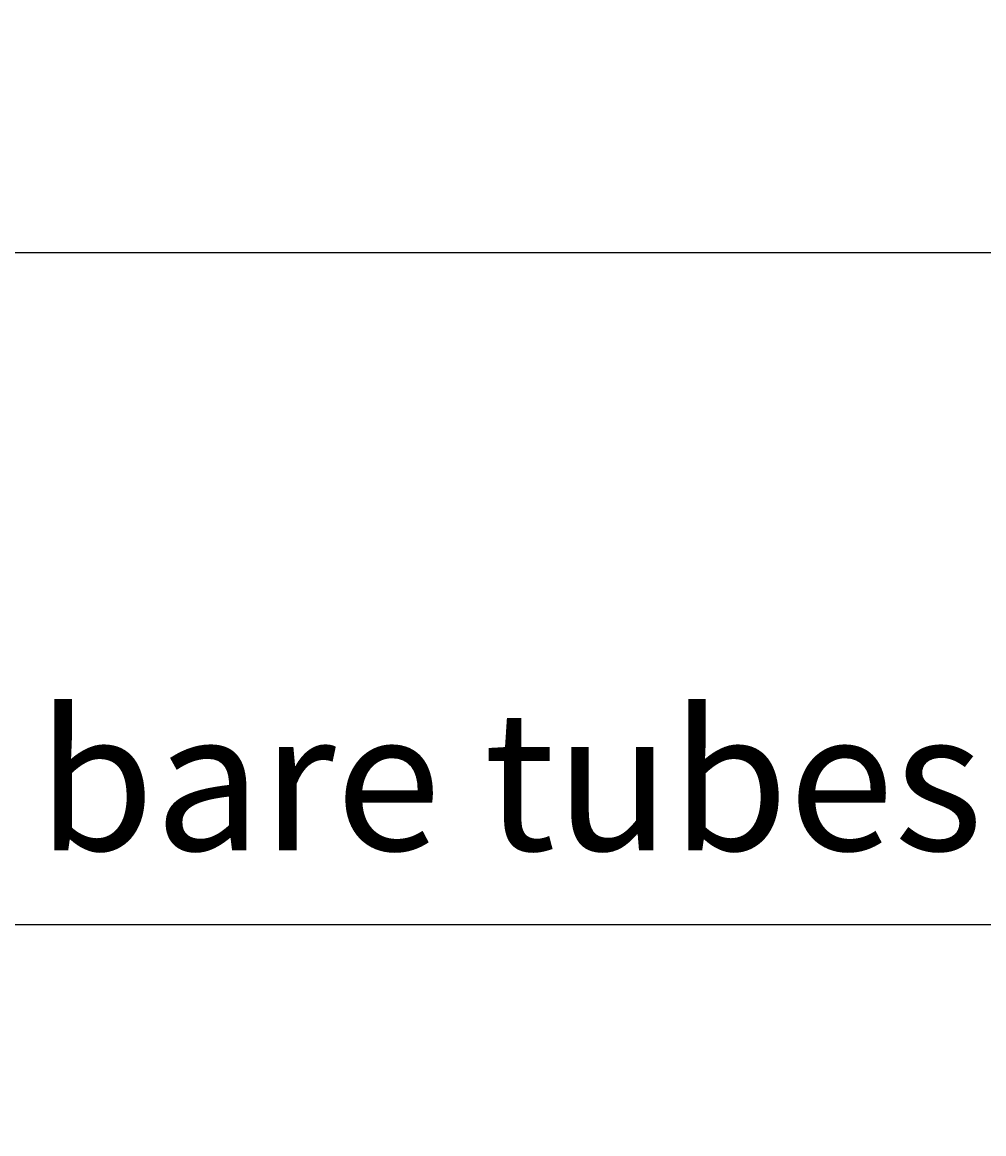
# Model space of a CAD drawing. Units: inches. Extents: x -1 to 292, y -3 to 199.
# Tile 3 of 52: x 25 to 46, y 21 to 45. Entities that reach past the tile are written whole.
import ezdxf

# ---------------------------------------------------------------- set-up
doc = ezdxf.new("R2010")
doc.units = ezdxf.units.IN
doc.header["$MEASUREMENT"] = 0
doc.layers.add('M-ANNO-TEXT', color=3, linetype='Continuous', lineweight=25)
doc.layers.add('M-DIMS', color=2, linetype='Continuous', lineweight=18)
doc.styles.get("Standard").update_dxf_attribs({"font": 'arial.ttf'})
doc.dimstyles.get("Standard").update_dxf_attribs({"dimtxt": 0.18, "dimasz": 0.18, "dimexe": 0.18, "dimexo": 0.0625, "dimgap": 0.09, "dimtad": 0, "dimtih": 1, "dimtoh": 1, "dimdec": 4, "dimzin": 0, "dimdsep": 46, "dimtxsty": 'Standard', "dimcen": 0.09, "dimadec": 0, "dimazin": 0, "dimtfac": 1, "dimtdec": 4, "dimtofl": 0, "dimtmove": 0, "dimatfit": 3, "dimfxl": 1, "dimtolj": 1, "dimtzin": 0, "dimarcsym": 0})

# ---------------------------------------------------------------- blocks, each defined once
blk = doc.blocks.new('*D7')
at = {"layer": 'Defpoints', "color": 0, "transparency": 16777216}
for p in [(21.861, 54.582), (205.115, 54.582), (21.861, 39.982)]:
    blk.add_point(p, dxfattribs=at)
at = {"layer": 'M-DIMS', "color": 0, "lineweight": -2, "transparency": 16777216}
for p, q in [((21.861, 54.52), (21.861, 39.802)), ((205.115, 54.52), (205.115, 39.802)), ((22.041, 39.982), (113.033, 39.982)), ((204.935, 39.982), (113.944, 39.982))]:
    blk.add_line(p, q, dxfattribs=at)
at = {"layer": 'M-DIMS', "color": 0, "transparency": 16777216}
for points in [[(22.041, 40.012), (22.041, 39.952), (21.861, 39.982)], [(204.935, 40.012), (204.935, 39.952), (205.115, 39.982)]]:
    blk.add_solid(points, dxfattribs=at)
at = {"layer": 'M-DIMS', "color": 0, "transparency": 16777216, "insert": (113.488, 39.982), "char_height": 0.18, "attachment_point": 5}
blk.add_mtext('\\A1;183.25', dxfattribs=at)
blk = doc.blocks.new('*D8')
at = {"layer": 'Defpoints', "color": 0, "transparency": 16777216}
for p in [(-0.662, 126.765), (111.488, 126.765), (69.013, 25.514)]:
    blk.add_point(p, dxfattribs=at)
at = {"layer": 'M-DIMS', "color": 0, "lineweight": -2, "transparency": 16777216}
for p, q in [((111.426, 126.765), (-0.842, 126.765)), ((-0.662, 126.585), (-0.662, 76.321)), ((-0.662, 25.694), (-0.662, 75.958)), ((68.951, 25.514), (-0.842, 25.514))]:
    blk.add_line(p, q, dxfattribs=at)
at = {"layer": 'M-DIMS', "color": 0, "transparency": 16777216}
for points in [[(-0.692, 126.585), (-0.632, 126.585), (-0.662, 126.765)], [(-0.692, 25.694), (-0.632, 25.694), (-0.662, 25.514)]]:
    blk.add_solid(points, dxfattribs=at)
at = {"layer": 'M-DIMS', "color": 0, "transparency": 16777216, "insert": (-0.662, 76.14), "char_height": 0.18, "attachment_point": 5}
blk.add_mtext('\\A1;101.25', dxfattribs=at)
blk = doc.blocks.new('*D23')
at = {"layer": 'Defpoints', "color": 0, "transparency": 16777216}
for p in [(21.861, 54.582), (64.679, 51.267), (64.679, -2.71)]:
    blk.add_point(p, dxfattribs=at)
at = {"layer": 'M-DIMS', "color": 0, "lineweight": -2, "transparency": 16777216}
for p, q in [((21.861, 54.52), (21.861, -2.89)), ((64.679, 51.205), (64.679, -2.89)), ((22.041, -2.71), (42.874, -2.71)), ((64.499, -2.71), (43.666, -2.71))]:
    blk.add_line(p, q, dxfattribs=at)
at = {"layer": 'M-DIMS', "color": 0, "transparency": 16777216}
for points in [[(22.041, -2.68), (22.041, -2.74), (21.861, -2.71)], [(64.499, -2.68), (64.499, -2.74), (64.679, -2.71)]]:
    blk.add_solid(points, dxfattribs=at)
at = {"layer": 'M-DIMS', "color": 0, "transparency": 16777216, "insert": (43.27, -2.71), "char_height": 0.18, "attachment_point": 5}
blk.add_mtext('\\A1;42.82', dxfattribs=at)

msp = doc.modelspace()

# ---------------------------------------------------------------- texts
at = {"layer": 'M-ANNO-TEXT', "insert": (25.6708, 30.1189), "char_height": 3, "attachment_point": 1}
msp.add_mtext_dynamic_manual_height_columns('bare tubes', width=47.899539, gutter_width=1, heights=[0], dxfattribs=at)

# ---------------------------------------------------------------- dimensions: what is measured, and where the dimension line sits
at = {"layer": 'M-DIMS'}
for base, p1, p2, angle, picture, middle in [((-0.6625, 126.765), (69.013, 25.5141), (111.4883, 126.765), 90, '*D8', (-0.6625, 76.1396)), ((21.8612, 39.9821), (205.1155, 54.5821), (21.8612, 54.5821), 180, '*D7', (113.4883, 39.9821))]:
    dim = msp.add_linear_dim(base=base, p1=p1, p2=p2, angle=angle, dimstyle='Standard', override={"dimdec": 2, "dimlfac": 1, "dimrnd": 0, "dimzin": 0, "dimdsep": 46, "dimlunit": 2}, dxfattribs=at)
    dim.commit()
    dim.dimension.update_dxf_attribs({"geometry": picture, "text_midpoint": middle})
dim = msp.add_linear_dim(base=(64.6788, -2.7104), p1=(21.8612, 54.5821), p2=(64.6788, 51.2672), dimstyle='Standard', override={"dimdec": 2, "dimlfac": 1, "dimrnd": 0, "dimzin": 0, "dimdsep": 46, "dimlunit": 2}, dxfattribs=at)
dim.commit()
dim.dimension.update_dxf_attribs({"geometry": '*D23', "text_midpoint": (43.27, -2.7104)})

doc.saveas('drawing.dxf')
